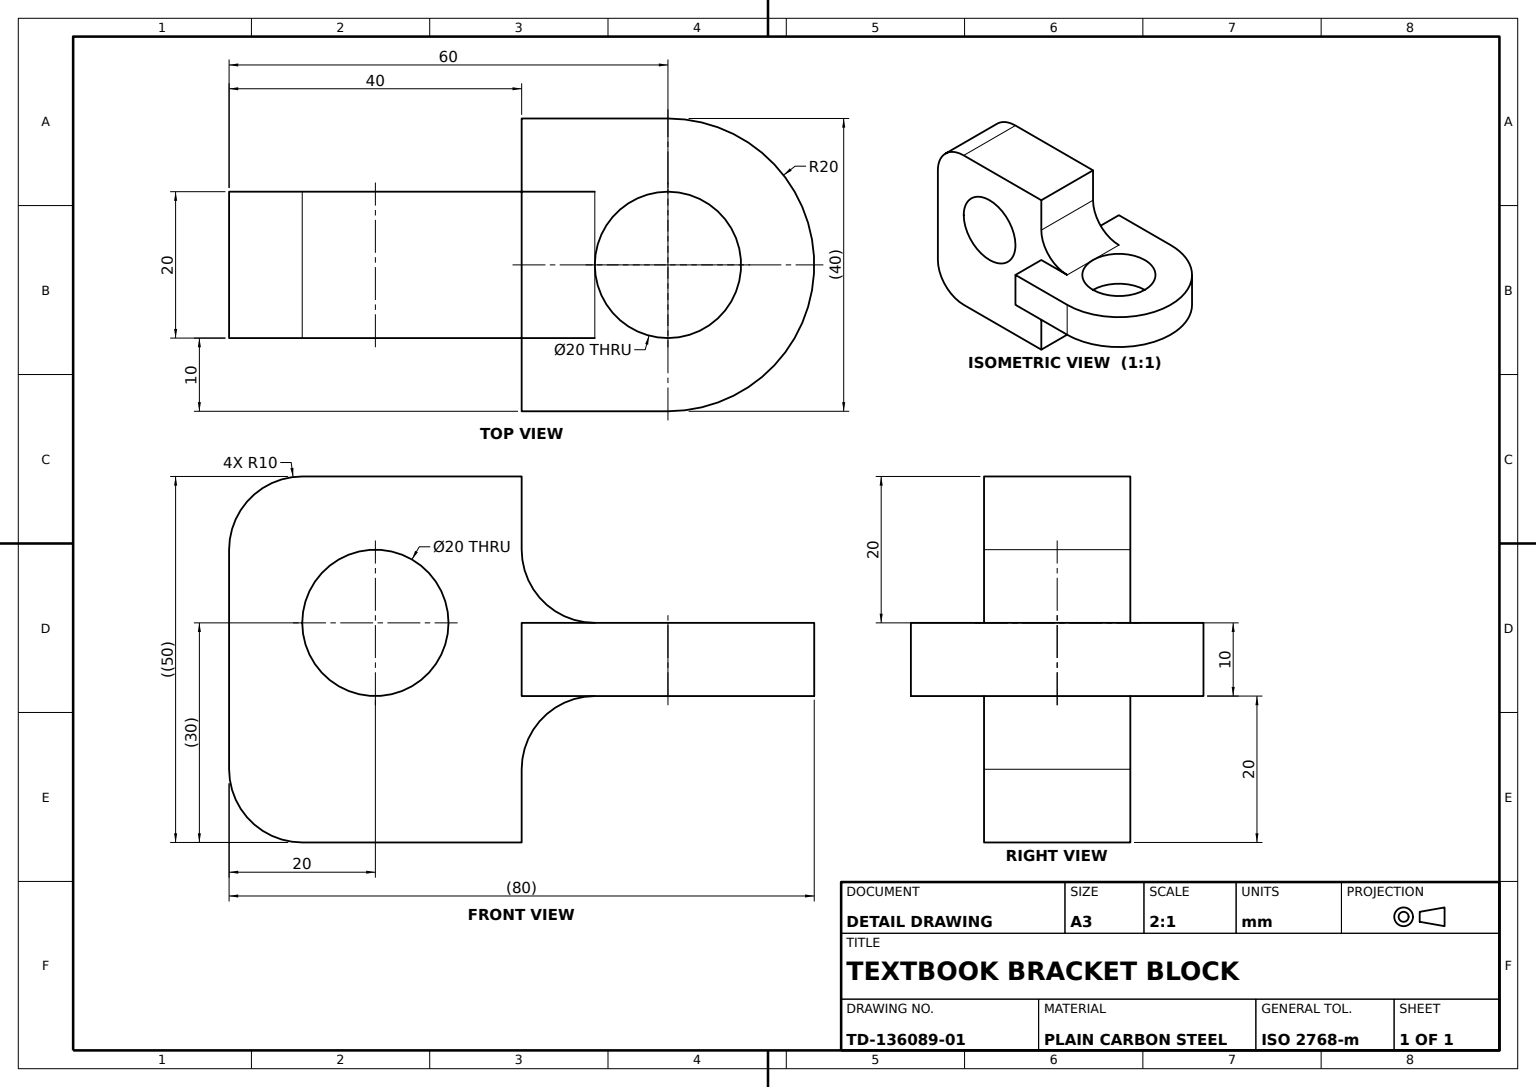
from build123d import *

# Parameters (mm, degrees)
BASE_BLOCK_DEPTH           = 10
LUG_TAB_PROFILE_W          = 40
LUG_TAB_PROFILE_H          = 40
LUG_TAB_DEPTH              = 5
LUG_TAB_EDGE_FILLET_RADIUS = 20
LUG_TAB_EDGE_FILLET_LENGTH = 10
CORNER_FILLET_R10_R        = 10
CROSS_HOLE_PROFILE_R       = 10
CROSS_HOLE_20_DEPTH        = 72.589105316
LUG_HOLE_PROFILE_R         = 10
LUG_HOLE_20_DEPTH          = 71


with BuildPart() as part:
    # Base Block Profile → Base Block (new, symmetric)
    with BuildSketch(Plane.XY):
        with BuildLine():
            Line((20, -25), (-10, -25))
            ThreePointArc((-10, -25), (-17.071067812, -22.071067812), (-20, -15))
            Line((-20, -15), (-20, 15))
            ThreePointArc((-20, 15), (-17.071067812, 22.071067812), (-10, 25))
            Line((-10, 25), (20, 25))
            Line((20, 25), (20, -25))
        make_face()
    extrude(amount=BASE_BLOCK_DEPTH, both=True)

    # Lug Tab Profile → Lug Tab (add, symmetric)
    with BuildSketch(Plane(origin=(0, 0, 0), x_dir=(1, 0, 0), z_dir=(0, 1, 0))):
        with Locations((40, 0)):
            Rectangle(LUG_TAB_PROFILE_W, LUG_TAB_PROFILE_H)
    extrude(amount=LUG_TAB_DEPTH, both=True)

    # Lug Tab Edge Fillet: full round fillet: the end face becomes a half cylinder, R = half its width
    lug_tab_edge_fillet_face = Plane((60, 0, 0), x_dir=(0, -1, 0), z_dir=(1, 0, 0))  # on the end face: x along it, z out of the body
    lug_tab_edge_fillet_slab = lug_tab_edge_fillet_face.offset(-LUG_TAB_EDGE_FILLET_RADIUS / 2) * Box(LUG_TAB_EDGE_FILLET_LENGTH, 2 * LUG_TAB_EDGE_FILLET_RADIUS, LUG_TAB_EDGE_FILLET_RADIUS, mode=Mode.PRIVATE)  # the body's end, R deep
    lug_tab_edge_fillet_round = Plane((40, 0, 0), x_dir=(1, 0, 0), z_dir=(0, -1, 0)) * Cylinder(LUG_TAB_EDGE_FILLET_RADIUS, LUG_TAB_EDGE_FILLET_LENGTH, mode=Mode.PRIVATE)  # its axis R under the face
    add(lug_tab_edge_fillet_slab - lug_tab_edge_fillet_round, mode=Mode.SUBTRACT)

    # Corner Fillet R10
    corner_fillet_r10_edges = [part.edges().sort_by_distance(p)[0] for p in [
        (20, 5, 0),
        (20, -5, 0),
    ]]
    fillet(corner_fillet_r10_edges, radius=CORNER_FILLET_R10_R)

    # Cross Hole Profile → Cross Hole _20 (cut, through all)
    with BuildSketch(Plane.XY.offset(10)):
        with Locations((0, 5)):
            Circle(CROSS_HOLE_PROFILE_R)
    extrude(amount=-CROSS_HOLE_20_DEPTH, mode=Mode.SUBTRACT)

    # Lug Hole Profile → Lug Hole _20 (cut, through all)
    with BuildSketch(Plane(origin=(0, 5, 0), x_dir=(1, 0, 0), z_dir=(0, 1, 0))):
        with Locations(Location((40, 0, 0), (0, 0, 180))):
            Circle(LUG_HOLE_PROFILE_R)
    extrude(amount=-LUG_HOLE_20_DEPTH, mode=Mode.SUBTRACT)


solid = part.part
